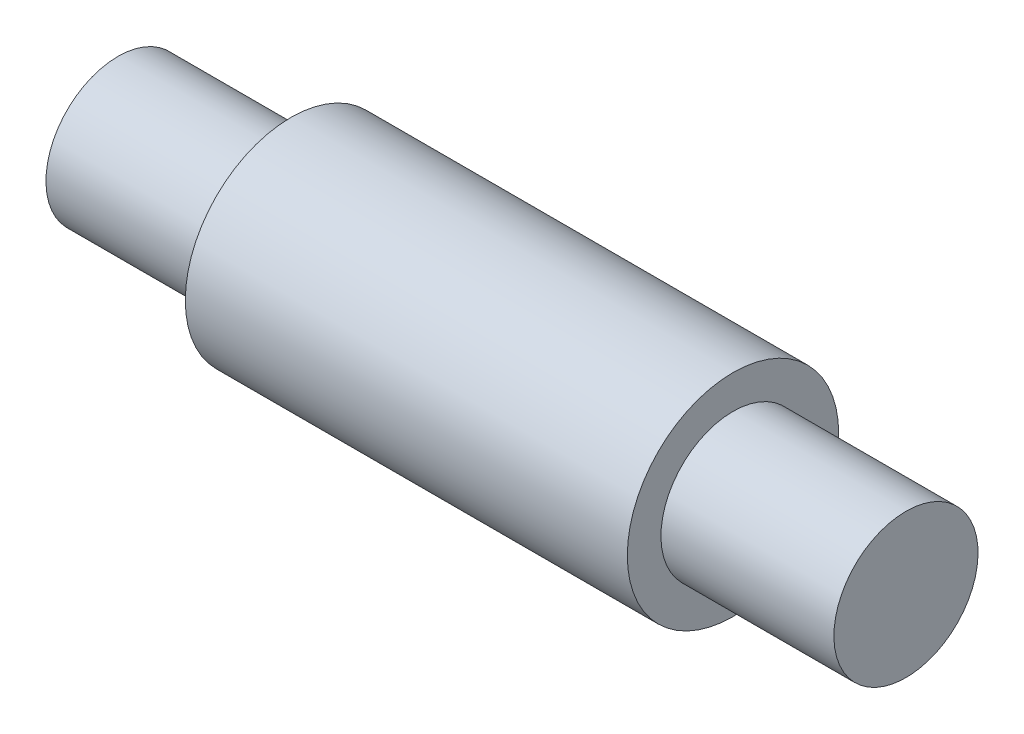
from build123d import *


with BuildPart() as part:
    # Spacer Profile Sketch → Spacer Body Revolve (revolve)
    with BuildSketch(Plane.XY):
        Polygon((-82, 0), (-82, 7.5), (-64, 7.5), (-64, 11), (-18, 11), (-18, 7.5), (0, 7.5), (0, 0), align=None)
    revolve(axis=Axis((0, 0, 0), (-1, 0, 0)))


solid = part.part
